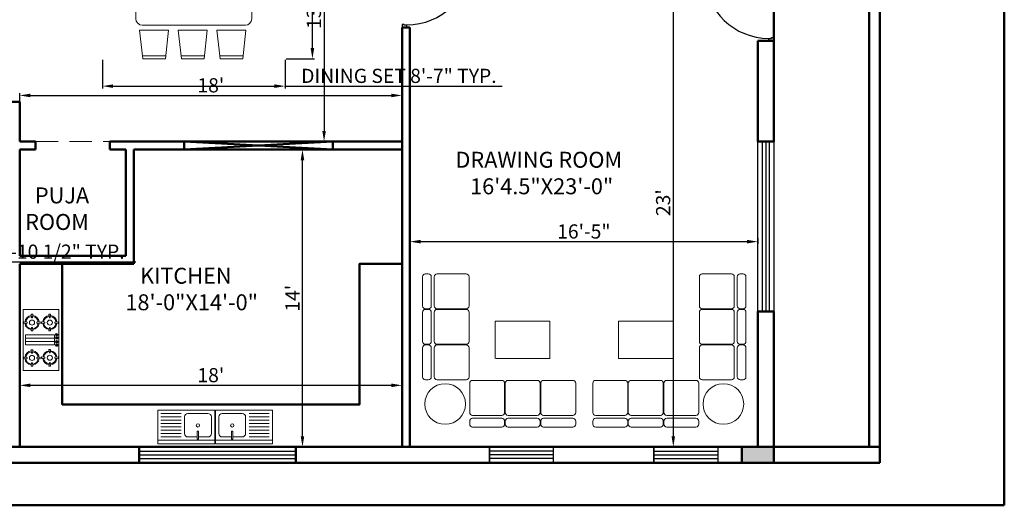
# Model space of a CAD drawing. Units: millimetres. Extents: x 1706 to 5913, y 156 to 1716.
# Tile 25 of 26: x 4935 to 5492, y 1141 to 1415. Entities that reach past the tile are written whole.
import ezdxf

# ---------------------------------------------------------------- set-up
doc = ezdxf.new("R2010")
doc.units = ezdxf.units.MM
doc.linetypes.add('DASHED', pattern=[19.05, 12.7, -6.35])
for name, color, linetype, lineweight in [('A-ANNO-DIMS', 2, 'Continuous', 18), ('A-AREA-IDEN', 3, 'Continuous', 18), ('A-COLS', 20, 'Continuous', 50), ('A-DOOR', 4, 'Continuous', 25), ('A-FLOR-OVHD', 9, 'DASHED', 18), ('A-FURN', 8, 'Continuous', 18), ('A-GLAZ', 150, 'Continuous', 25), ('A-WALL', 7, 'Continuous', 50)]:
    doc.layers.add(name, color=color, linetype=linetype, lineweight=lineweight)
doc.styles.get("Standard").update_dxf_attribs({"font": 'arial.ttf'})
doc.dimstyles.new('ISO-25', dxfattribs={"dimtxt": 8, "dimasz": 6, "dimexe": 1.25, "dimexo": 0.625, "dimtad": 1, "dimdec": 0, "dimlunit": 3, "dimtxsty": 'Standard', "dimcen": 2.5, "dimadec": 0, "dimazin": 0, "dimtfac": 1, "dimtdec": 0, "dimtmove": 0, "dimatfit": 3, "dimfxl": 1, "dimarcsym": 0})

# ---------------------------------------------------------------- blocks, each defined once
blk = doc.blocks.new('Puerta 01')
for p, q in [((-0.775, -0.026), (-0.737, -0.058)), ((-0.775, -0.058), (-0.737, -0.026)), ((-0.737, -0.058), (-0.737, -0.026)), ((-0.028, -0.058), (-0.066, -0.026)), ((-0.028, -0.026), (-0.066, -0.058)), ((-0.066, -0.058), (-0.066, -0.026))]:
    blk.add_line(p, q)
for points in [[(-0.028, 0), (-0.028, -0.026), (0.004, -0.026), (0.004, -0.036), (0.028, -0.036), (0.028, 0)], [(-0.028, -0.026), (-0.775, -0.026), (-0.775, -0.058), (-0.028, -0.058)], [(0.004, -0.774), (0.004, -0.764), (0.028, -0.764), (0.028, -0.8), (-0.028, -0.8), (-0.028, -0.774)]]:
    blk.add_lwpolyline(points, close=True)
blk.add_arc((-0.028, -0.026), 0.747, 182.4545, 270)
blk = doc.blocks.new('A$C57CF26DA')
for p, q in [((0, 0), (0, 420)), ((720, 420), (0, 420)), ((167, 413), (147, 413)), ((147, 413), (152, 373)), ((152, 373), (162, 373)), ((162, 373), (167, 413)), ((300, 391), (300, 49)), ((300, 391), (420, 391)), ((340, 391), (340, 49)), ((380, 391), (380, 49)), ((420, 391), (420, 49)), ((584, 413), (564, 413)), ((564, 413), (569, 373)), ((569, 373), (579, 373)), ((579, 373), (584, 413)), ((720, 0), (720, 420)), ((99, 320), (59, 325)), ((59, 325), (59, 305)), ((59, 305), (99, 310)), ((99, 310), (99, 320)), ((152, 257), (147, 217)), ((162, 257), (152, 257)), ((167, 217), (162, 257)), ((255, 325), (215, 320)), ((215, 320), (215, 310)), ((215, 310), (255, 305)), ((255, 305), (255, 325)), ((516, 320), (476, 325)), ((476, 325), (476, 305)), ((476, 305), (516, 310)), ((516, 310), (516, 320)), ((569, 257), (564, 217)), ((579, 257), (569, 257)), ((584, 217), (579, 257)), ((672, 325), (632, 320)), ((632, 320), (632, 310)), ((632, 310), (672, 305)), ((672, 305), (672, 325)), ((147, 217), (167, 217)), ((167, 203), (147, 203)), ((147, 203), (152, 163)), ((152, 163), (162, 163)), ((162, 163), (167, 203)), ((581, 203), (561, 203)), ((561, 203), (566, 163)), ((564, 217), (584, 217)), ((566, 163), (576, 163)), ((576, 163), (581, 203)), ((99, 110), (59, 115)), ((59, 115), (59, 95)), ((59, 95), (99, 100)), ((99, 100), (99, 110)), ((152, 47), (147, 7)), ((147, 7), (167, 7)), ((162, 47), (152, 47)), ((167, 7), (162, 47)), ((255, 115), (215, 110)), ((215, 110), (215, 100)), ((215, 100), (255, 95)), ((255, 95), (255, 115)), ((302, 39), (295, 39)), ((295, 39), (295, 11)), ((295, 11), (302, 11)), ((420, 49), (300, 49)), ((302, 11), (302, 39)), ((341, 39), (334, 39)), ((334, 39), (334, 11)), ((334, 11), (341, 11)), ((341, 11), (341, 39)), ((380, 11), (380, 39)), ((380, 39), (386, 39)), ((386, 11), (380, 11)), ((386, 39), (386, 11)), ((419, 11), (419, 39)), ((419, 39), (426, 39)), ((426, 11), (419, 11)), ((426, 39), (426, 11)), ((513, 110), (473, 115)), ((473, 115), (473, 95)), ((473, 95), (513, 100)), ((513, 100), (513, 110)), ((566, 47), (561, 7)), ((561, 7), (581, 7)), ((576, 47), (566, 47)), ((581, 7), (576, 47)), ((669, 115), (629, 110)), ((629, 110), (629, 100)), ((629, 100), (669, 95)), ((669, 95), (669, 115)), ((720, 0), (0, 0))]:
    blk.add_line(p, q)
for centre in [(157, 315), (574, 315), (157, 105), (571, 105)]:
    blk.add_circle(centre, 30)
for centre, radius, start, end in [((157, 315), 83, 95.5849, 174.4151), ((157, 315), 73, 95.3738, 174.6262), ((157, 315), 73, 5.3738, 84.6262), ((157, 315), 83, 5.5849, 84.4151), ((574, 315), 83, 95.5849, 174.4151), ((574, 315), 73, 95.3738, 174.6262), ((574, 315), 73, 5.3738, 84.6262), ((574, 315), 83, 5.5849, 84.4151), ((157, 315), 83, 185.5849, 264.4151), ((157, 315), 73, 185.3738, 264.6262), ((157, 315), 73, 275.3738, 354.6262), ((157, 315), 83, 275.5849, 354.4151), ((574, 315), 83, 185.5849, 264.4151), ((574, 315), 73, 185.3738, 264.6262), ((574, 315), 73, 275.3738, 354.6262), ((574, 315), 83, 275.5849, 354.4151), ((157, 105), 83, 95.5849, 174.4151), ((157, 105), 73, 95.3738, 174.6262), ((157, 105), 73, 5.3738, 84.6262), ((157, 105), 83, 5.5849, 84.4151), ((571, 105), 83, 95.5849, 174.4151), ((571, 105), 73, 95.3738, 174.6262), ((571, 105), 73, 5.3738, 84.6262), ((571, 105), 83, 5.5849, 84.4151), ((157, 105), 83, 185.5849, 264.4151), ((157, 105), 73, 185.3738, 264.6262), ((157, 105), 73, 275.3738, 354.6262), ((157, 105), 83, 275.5849, 354.4151), ((298, 25), 13.7, 104.4775, 255.5225), ((298, 25), 13.7, 284.4775, 75.5225), ((337, 25), 13.7, 104.4775, 255.5225), ((337, 25), 13.7, 284.4775, 75.5225), ((383, 25), 13.7, 104.4775, 255.5225), ((383, 25), 13.7, 284.4775, 75.5225), ((422, 25), 13.7, 104.4775, 255.5225), ((422, 25), 13.7, 284.4775, 75.5225), ((571, 105), 83, 185.5849, 264.4151), ((571, 105), 73, 185.3738, 264.6262), ((571, 105), 73, 275.3738, 354.6262), ((571, 105), 83, 275.5849, 354.4151)]:
    blk.add_arc(centre, radius, start, end)
blk = doc.blocks.new('A$C3404121D')
for p, q in [((0, 0), (0, 500)), ((0, 500), (850, 500)), ((0, 450), (850, 450)), ((850, 500), (850, 0)), ((50, 100), (50, 350)), ((100, 400), (240, 400)), ((240, 431), (240, 425)), ((260, 431), (240, 431)), ((240, 425), (240, 315)), ((240, 315), (260, 315)), ((260, 431), (260, 315)), ((260, 400), (400, 400)), ((450, 100), (450, 350)), ((502, 400), (801, 400)), ((502, 350), (801, 350)), ((502, 300), (801, 300)), ((502, 250), (801, 250)), ((502, 200), (801, 200)), ((502, 150), (801, 150)), ((850, 0), (0, 0)), ((400, 50), (100, 50)), ((502, 100), (801, 100)), ((801, 50), (502, 50))]:
    blk.add_line(p, q)
blk.add_circle((250, 228), 25)
for centre, start, end in [((100, 350), 90, 180), ((400, 350), 0, 90), ((100, 100), 180, 270), ((400, 100), 270, 0)]:
    blk.add_arc(centre, 50, start, end)
blk = doc.blocks.new('A$C59D7588A')
for p, q in [((0.575, 1.5), (0.623, 1.943)), ((0.618, 1.9), (0.982, 1.9)), ((0.623, 1.943), (0.978, 1.943)), ((0.978, 1.943), (1.025, 1.5)), ((1.175, 1.5), (1.223, 1.943)), ((1.218, 1.9), (1.582, 1.9)), ((1.223, 1.943), (1.578, 1.943)), ((1.578, 1.943), (1.625, 1.5)), ((1.775, 1.5), (1.823, 1.943)), ((1.818, 1.9), (2.182, 1.9)), ((1.823, 1.943), (2.178, 1.943)), ((2.178, 1.943), (2.225, 1.5)), ((1.025, 1.5), (0.575, 1.5)), ((0.616, 1.421), (2.216, 1.421)), ((1.625, 1.5), (1.175, 1.5)), ((2.225, 1.5), (1.775, 1.5)), ((0.516, 0.621), (0.516, 1.321)), ((2.316, 1.321), (2.316, 0.621)), ((0, 1.146), (0.443, 1.194)), ((0, 0.792), (0, 1.146)), ((0.043, 0.787), (0.043, 1.151)), ((0.443, 1.194), (0.443, 0.744)), ((2.832, 1.146), (2.389, 1.194)), ((2.389, 1.194), (2.389, 0.744)), ((2.789, 0.787), (2.789, 1.151)), ((2.832, 0.792), (2.832, 1.146)), ((0.443, 0.744), (0, 0.792)), ((2.389, 0.744), (2.832, 0.792)), ((2.216, 0.521), (0.616, 0.521)), ((1.025, 0.443), (0.575, 0.443)), ((0.575, 0.443), (0.623, 0)), ((0.978, 0), (1.025, 0.443)), ((1.625, 0.443), (1.175, 0.443)), ((1.175, 0.443), (1.223, 0)), ((1.578, 0), (1.625, 0.443)), ((2.225, 0.443), (1.775, 0.443)), ((1.775, 0.443), (1.823, 0)), ((2.178, 0), (2.225, 0.443)), ((0.618, 0.043), (0.982, 0.043)), ((1.218, 0.043), (1.582, 0.043)), ((1.818, 0.043), (2.182, 0.043)), ((0.623, 0), (0.978, 0)), ((1.223, 0), (1.578, 0)), ((1.823, 0), (2.178, 0))]:
    blk.add_line(p, q)
for centre, start, end in [((0.616, 1.321), 90, 180), ((2.216, 1.321), 0, 90), ((0.616, 0.621), 180, 270), ((2.216, 0.621), 270, 0)]:
    blk.add_arc(centre, 0.1, start, end)
blk = doc.blocks.new('A$C753D6792')
at = {"linetype": 'ByBlock'}
for p, q in [((0, 2530), (0, 2580)), ((50, 2630), (550, 2630)), ((600, 2580), (600, 2530)), ((610, 2530), (610, 2580)), ((660, 2630), (1160, 2630)), ((1210, 2580), (1210, 2530)), ((1220, 2530), (1220, 2580)), ((1270, 2630), (1770, 2630)), ((1820, 2580), (1820, 2530)), ((0, 1880), (0, 2380)), ((550, 2480), (50, 2480)), ((550, 2430), (50, 2430)), ((600, 2380), (600, 1880)), ((610, 1880), (610, 2380)), ((1160, 2480), (660, 2480)), ((1160, 2430), (660, 2430)), ((1210, 2380), (1210, 1880)), ((1220, 1880), (1220, 2380)), ((1770, 2480), (1270, 2480)), ((1770, 2430), (1270, 2430)), ((1820, 1880), (1820, 2380)), ((50, 1830), (427, 1830)), ((387, 1830), (550, 1830)), ((660, 1830), (1037, 1830)), ((997, 1830), (1160, 1830)), ((1270, 1830), (1647, 1830)), ((1607, 1830), (1770, 1830)), ((1830, 1770), (1830, 1393)), ((1880, 1820), (2380, 1820)), ((2430, 1270), (2430, 1770)), ((2480, 1270), (2480, 1770)), ((2530, 1820), (2580, 1820)), ((2630, 1770), (2630, 1270)), ((442, 815), (442, 1455)), ((442, 1455), (1372, 1455)), ((1382, 1455), (1382, 815)), ((1830, 1433), (1830, 1270)), ((2380, 1220), (1880, 1220)), ((1880, 1210), (2380, 1210)), ((2580, 1220), (2530, 1220)), ((2530, 1210), (2580, 1210)), ((1830, 1160), (1830, 783)), ((2430, 660), (2430, 1160)), ((2480, 660), (2480, 1160)), ((2630, 1160), (2630, 660)), ((1382, 815), (442, 815)), ((1830, 823), (1830, 660)), ((1830, 550), (1830, 173)), ((2380, 610), (1880, 610)), ((1880, 600), (2380, 600)), ((2430, 50), (2430, 550)), ((2480, 50), (2480, 550)), ((2580, 610), (2530, 610)), ((2530, 600), (2580, 600)), ((2630, 550), (2630, 50)), ((1830, 213), (1830, 50)), ((2380, 0), (1880, 0)), ((2580, 0), (2530, 0))]:
    blk.add_line(p, q, dxfattribs=at)
blk.add_circle((2242, 2235), 349, dxfattribs=at)
for centre, start, end in [((50, 2580), 90, 180), ((550, 2580), 0, 90), ((550, 2580), 0, 90), ((660, 2580), 90, 180), ((1160, 2580), 0, 90), ((1160, 2580), 0, 90), ((1270, 2580), 90, 180), ((1770, 2580), 0, 90), ((1770, 2580), 0, 90), ((50, 2530), 180, 270), ((50, 2380), 90, 180), ((550, 2530), 270, 0), ((550, 2530), 270, 0), ((550, 2380), 0, 90), ((550, 2380), 0, 90), ((660, 2530), 180, 270), ((660, 2380), 90, 180), ((1160, 2530), 270, 0), ((1160, 2530), 270, 0), ((1160, 2380), 0, 90), ((1160, 2380), 0, 90), ((1270, 2530), 180, 270), ((1270, 2380), 90, 180), ((1770, 2530), 270, 0), ((1770, 2530), 270, 0), ((1770, 2380), 0, 90), ((1770, 2380), 0, 90), ((50, 1880), 180, 270), ((550, 1880), 270, 0), ((660, 1880), 180, 270), ((1160, 1880), 270, 0), ((1270, 1880), 180, 270), ((1770, 1880), 270, 0), ((1880, 1770), 90, 180), ((2380, 1770), 0, 90), ((2530, 1770), 90, 180), ((2580, 1770), 0, 90), ((1880, 1270), 180, 270), ((1880, 1160), 90, 180), ((2380, 1270), 270, 0), ((2380, 1270), 270, 0), ((2380, 1160), 0, 90), ((2530, 1270), 180, 270), ((2530, 1270), 180, 270), ((2530, 1160), 90, 180), ((2580, 1270), 270, 0), ((2580, 1270), 270, 0), ((2580, 1160), 0, 90), ((1880, 660), 180, 270), ((1880, 550), 90, 180), ((2380, 660), 270, 0), ((2380, 660), 270, 0), ((2380, 550), 0, 90), ((2530, 660), 180, 270), ((2530, 660), 180, 270), ((2530, 550), 90, 180), ((2580, 660), 270, 0), ((2580, 660), 270, 0), ((2580, 550), 0, 90), ((1880, 50), 180, 270), ((2380, 50), 270, 0), ((2380, 50), 270, 0), ((2530, 50), 180, 270), ((2530, 50), 180, 270), ((2580, 50), 270, 0), ((2580, 50), 270, 0)]:
    blk.add_arc(centre, 50, start, end, dxfattribs=at)
blk = doc.blocks.new('*D68')
at = {"layer": 'A-ANNO-DIMS', "color": 0, "lineweight": -2, "transparency": 16777216}
for p, q in [((5104.76, 1503.68), (5108.61, 1503.68)), ((5107.36, 1497.68), (5107.36, 1352.18)), ((5104.76, 1346.18), (5108.61, 1346.18))]:
    blk.add_line(p, q, dxfattribs=at)
at = {"layer": 'A-ANNO-DIMS', "color": 0, "transparency": 16777216}
for points in [[(5106.36, 1497.68), (5108.36, 1497.68), (5107.36, 1503.68)], [(5106.36, 1352.18), (5108.36, 1352.18), (5107.36, 1346.18)]]:
    blk.add_solid(points, dxfattribs=at)
at = {"layer": 'Defpoints', "color": 0, "transparency": 16777216}
for p in [(5104.13, 1503.68), (5104.13, 1346.18), (5107.36, 1346.18)]:
    blk.add_point(p, dxfattribs=at)
at = {"layer": 'A-ANNO-DIMS', "color": 0, "transparency": 16777216, "insert": (5102.64, 1424.93), "char_height": 8, "attachment_point": 5, "rotation": 90}
blk.add_mtext('13\'-2"', dxfattribs=at)
blk = doc.blocks.new('*D69')
at = {"layer": 'A-ANNO-DIMS', "color": 0, "lineweight": -2, "transparency": 16777216}
for p, q in [((4935.38, 1359.93), (4935.38, 1373.5)), ((4941.38, 1372.25), (5145.38, 1372.25)), ((5151.38, 1359.93), (5151.38, 1373.5))]:
    blk.add_line(p, q, dxfattribs=at)
at = {"layer": 'A-ANNO-DIMS', "color": 0, "transparency": 16777216}
for points in [[(4941.38, 1373.25), (4941.38, 1371.25), (4935.38, 1372.25)], [(5145.38, 1373.25), (5145.38, 1371.25), (5151.38, 1372.25)]]:
    blk.add_solid(points, dxfattribs=at)
at = {"layer": 'Defpoints', "color": 0, "transparency": 16777216}
for p in [(5151.38, 1372.25), (4935.38, 1359.3), (5151.38, 1359.3)]:
    blk.add_point(p, dxfattribs=at)
at = {"layer": 'A-ANNO-DIMS', "color": 0, "transparency": 16777216, "insert": (5043.38, 1376.96), "char_height": 8, "attachment_point": 5}
blk.add_mtext("18'", dxfattribs=at)
blk = doc.blocks.new('*D70')
at = {"layer": 'A-ANNO-DIMS', "color": 0, "lineweight": -2, "transparency": 16777216}
for p, q in [((5096.14, 1341.68), (5093.9, 1341.68)), ((5095.15, 1179.68), (5095.15, 1335.68)), ((5096.14, 1173.68), (5093.9, 1173.68))]:
    blk.add_line(p, q, dxfattribs=at)
at = {"layer": 'A-ANNO-DIMS', "color": 0, "transparency": 16777216}
for points in [[(5094.15, 1335.68), (5096.15, 1335.68), (5095.15, 1341.68)], [(5094.15, 1179.68), (5096.15, 1179.68), (5095.15, 1173.68)]]:
    blk.add_solid(points, dxfattribs=at)
at = {"layer": 'Defpoints', "color": 0, "transparency": 16777216}
for p in [(5095.15, 1341.68), (5096.77, 1341.68), (5096.77, 1173.68)]:
    blk.add_point(p, dxfattribs=at)
at = {"layer": 'A-ANNO-DIMS', "color": 0, "transparency": 16777216, "insert": (5090.51, 1257.68), "char_height": 8, "attachment_point": 5, "rotation": 90}
blk.add_mtext("14'", dxfattribs=at)
blk = doc.blocks.new('*D71')
at = {"layer": 'A-ANNO-DIMS', "color": 0, "lineweight": -2, "transparency": 16777216}
for p, q in [((4935.38, 1201.14), (4935.38, 1209.73)), ((4941.38, 1208.48), (5145.38, 1208.48)), ((5151.38, 1201.14), (5151.38, 1209.73))]:
    blk.add_line(p, q, dxfattribs=at)
at = {"layer": 'A-ANNO-DIMS', "color": 0, "transparency": 16777216}
for points in [[(4941.38, 1209.48), (4941.38, 1207.48), (4935.38, 1208.48)], [(5145.38, 1209.48), (5145.38, 1207.48), (5151.38, 1208.48)]]:
    blk.add_solid(points, dxfattribs=at)
at = {"layer": 'Defpoints', "color": 0, "transparency": 16777216}
for p in [(5151.38, 1208.48), (4935.38, 1200.51), (5151.38, 1200.51)]:
    blk.add_point(p, dxfattribs=at)
at = {"layer": 'A-ANNO-DIMS', "color": 0, "transparency": 16777216, "insert": (5043.38, 1213.19), "char_height": 8, "attachment_point": 5}
blk.add_mtext("18'", dxfattribs=at)
blk = doc.blocks.new('*D72')
at = {"layer": 'A-ANNO-DIMS', "color": 0, "lineweight": -2, "transparency": 16777216}
for p, q in [((5301.19, 1449.68), (5305.91, 1449.68)), ((5304.66, 1443.68), (5304.66, 1179.68)), ((5301.19, 1173.68), (5305.91, 1173.68))]:
    blk.add_line(p, q, dxfattribs=at)
at = {"layer": 'A-ANNO-DIMS', "color": 0, "transparency": 16777216}
for points in [[(5303.66, 1443.68), (5305.66, 1443.68), (5304.66, 1449.68)], [(5303.66, 1179.68), (5305.66, 1179.68), (5304.66, 1173.68)]]:
    blk.add_solid(points, dxfattribs=at)
at = {"layer": 'Defpoints', "color": 0, "transparency": 16777216}
for p in [(5300.56, 1449.68), (5300.56, 1173.68), (5304.66, 1173.68)]:
    blk.add_point(p, dxfattribs=at)
at = {"layer": 'A-ANNO-DIMS', "color": 0, "transparency": 16777216, "insert": (5299.95, 1311.68), "char_height": 8, "attachment_point": 5, "rotation": 90}
blk.add_mtext("23'", dxfattribs=at)
blk = doc.blocks.new('*D73')
at = {"layer": 'A-ANNO-DIMS', "color": 0, "lineweight": -2, "transparency": 16777216}
for p, q in [((5155.88, 1291.56), (5155.88, 1288.41)), ((5352.38, 1291.56), (5352.38, 1288.41)), ((5161.88, 1289.66), (5346.38, 1289.66))]:
    blk.add_line(p, q, dxfattribs=at)
at = {"layer": 'A-ANNO-DIMS', "color": 0, "transparency": 16777216}
for points in [[(5161.88, 1290.66), (5161.88, 1288.66), (5155.88, 1289.66)], [(5346.38, 1290.66), (5346.38, 1288.66), (5352.38, 1289.66)]]:
    blk.add_solid(points, dxfattribs=at)
at = {"layer": 'Defpoints', "color": 0, "transparency": 16777216}
for p in [(5155.88, 1292.18), (5352.38, 1292.18), (5352.38, 1289.66)]:
    blk.add_point(p, dxfattribs=at)
at = {"layer": 'A-ANNO-DIMS', "color": 0, "transparency": 16777216, "insert": (5254.13, 1294.37), "char_height": 8, "attachment_point": 5}
blk.add_mtext('16\'-5"', dxfattribs=at)
blk = doc.blocks.new('*D215')
at = {"layer": 'A-ANNO-DIMS', "color": 0, "lineweight": -2, "transparency": 16777216}
for p, q in [((4692.95, 1264.63), (4692.95, 1279.45)), ((4698.95, 1278.2), (4781.6, 1278.2)), ((4787.6, 1264.63), (4787.6, 1279.45)), ((4787.6, 1278.2), (5001.01, 1278.2))]:
    blk.add_line(p, q, dxfattribs=at)
at = {"layer": 'A-ANNO-DIMS', "color": 0, "transparency": 16777216}
for points in [[(4698.95, 1279.2), (4698.95, 1277.2), (4692.95, 1278.2)], [(4781.6, 1279.2), (4781.6, 1277.2), (4787.6, 1278.2)]]:
    blk.add_solid(points, dxfattribs=at)
at = {"layer": 'Defpoints', "color": 0, "transparency": 16777216}
for p in [(4787.6, 1278.2), (4692.95, 1264.01), (4787.6, 1264.01)]:
    blk.add_point(p, dxfattribs=at)
at = {"layer": 'A-ANNO-DIMS', "color": 0, "transparency": 16777216, "insert": (4897.3, 1282.96), "char_height": 8, "attachment_point": 5}
blk.add_mtext('BED WITH SIDE TABLES 7\'-10 1/2" TYP.', dxfattribs=at)
blk = doc.blocks.new('*D231')
at = {"layer": 'A-ANNO-DIMS', "color": 0, "lineweight": -2, "transparency": 16777216}
for p, q in [((4982.19, 1392.37), (4982.19, 1376.27)), ((5085.29, 1392.37), (5085.29, 1376.27)), ((4988.19, 1377.52), (5079.29, 1377.52)), ((5085.29, 1377.52), (5207.97, 1377.52))]:
    blk.add_line(p, q, dxfattribs=at)
at = {"layer": 'A-ANNO-DIMS', "color": 0, "transparency": 16777216}
for points in [[(4988.19, 1378.52), (4988.19, 1376.52), (4982.19, 1377.52)], [(5079.29, 1378.52), (5079.29, 1376.52), (5085.29, 1377.52)]]:
    blk.add_solid(points, dxfattribs=at)
at = {"layer": 'Defpoints', "color": 0, "transparency": 16777216}
for p in [(4982.19, 1392.99), (5085.29, 1392.99), (5085.29, 1377.52)]:
    blk.add_point(p, dxfattribs=at)
at = {"layer": 'A-ANNO-DIMS', "color": 0, "transparency": 16777216, "insert": (5149.63, 1382.29), "char_height": 8, "attachment_point": 5}
blk.add_mtext('DINING SET 8\'-7" TYP.', dxfattribs=at)
blk = doc.blocks.new('*D232')
at = {"layer": 'A-ANNO-DIMS', "color": 0, "lineweight": -2, "transparency": 16777216}
for p, q in [((5100.76, 1463.72), (5100.76, 1544.6)), ((5085.92, 1463.72), (5102.01, 1463.72)), ((5100.76, 1398.99), (5100.76, 1457.72)), ((5085.92, 1392.99), (5102.01, 1392.99))]:
    blk.add_line(p, q, dxfattribs=at)
at = {"layer": 'A-ANNO-DIMS', "color": 0, "transparency": 16777216}
for points in [[(5099.76, 1457.72), (5101.76, 1457.72), (5100.76, 1463.72)], [(5099.76, 1398.99), (5101.76, 1398.99), (5100.76, 1392.99)]]:
    blk.add_solid(points, dxfattribs=at)
at = {"layer": 'Defpoints', "color": 0, "transparency": 16777216}
for p in [(5085.29, 1463.72), (5100.76, 1463.72), (5085.29, 1392.99)]:
    blk.add_point(p, dxfattribs=at)
at = {"layer": 'A-ANNO-DIMS', "color": 0, "transparency": 16777216, "insert": (5096, 1507.16), "char_height": 8, "attachment_point": 5, "rotation": 90}
blk.add_mtext('5\'-10 1/2" TYP.', dxfattribs=at)

msp = doc.modelspace()

# ---------------------------------------------------------------- hatches: boundary and pattern name
at = {"layer": 'A-COLS'}
h = msp.add_hatch(color=256, dxfattribs=at)
h.dxf.hatch_style = 1
h.paths.add_polyline_path([(5361.38, 1173.68), (5343.38, 1173.68), (5343.38, 1164.68), (5361.38, 1164.68)])

# ---------------------------------------------------------------- linework, layer by layer
msp.add_lwpolyline([(5361.6, 1173.68), (5343.38, 1173.68), (5343.38, 1164.68), (5361.38, 1164.68), (5361.38, 1173.68)], dxfattribs=at)
at = {"layer": 'A-FLOR-OVHD'}
msp.add_line((4944.38, 1346.18), (4986.38, 1346.18), dxfattribs=at)
at = {"layer": 'A-GLAZ'}
for p, q in [((5354.88, 1346.18), (5354.88, 1250.18)), ((5356.88, 1346.18), (5356.88, 1250.18)), ((5358.88, 1346.18), (5358.88, 1250.18)), ((5002.88, 1171.18), (5091.38, 1171.18)), ((5002.88, 1169.18), (5091.38, 1169.18)), ((5200.74, 1173.68), (5200.74, 1164.68)), ((5236.74, 1171.18), (5200.74, 1171.18)), ((5236.74, 1169.18), (5200.74, 1169.18)), ((5236.74, 1173.68), (5236.74, 1164.68)), ((5293.74, 1173.68), (5293.74, 1164.68)), ((5293.74, 1171.18), (5329.74, 1171.18)), ((5293.74, 1169.18), (5329.74, 1169.18)), ((5329.74, 1173.68), (5329.74, 1164.68)), ((5002.88, 1167.18), (5091.38, 1167.18)), ((5236.74, 1167.18), (5200.74, 1167.18)), ((5293.74, 1167.18), (5329.74, 1167.18))]:
    msp.add_line(p, q, dxfattribs=at)
for points in [[(5352.38, 1346.18), (5361.38, 1346.18), (5361.38, 1250.18), (5352.38, 1250.18)], [(5002.88, 1173.68), (5091.38, 1173.68), (5091.38, 1164.68), (5002.88, 1164.68)], [(5200.74, 1173.68), (5236.74, 1173.68), (5236.74, 1164.68), (5200.74, 1164.68)], [(5293.74, 1173.68), (5329.74, 1173.68), (5329.74, 1164.68), (5293.74, 1164.68)]]:
    msp.add_lwpolyline(points, close=True, dxfattribs=at)
at = {"layer": 'A-WALL'}
for p, q in [((5491.67, 1664.18), (5491.67, 1140.68)), ((5415.38, 1655.18), (5415.38, 1173.68)), ((5421.38, 1655.18), (5421.38, 1173.68)), ((5361.38, 1442.18), (5361.38, 1403.18)), ((5151.38, 1410.68), (5151.38, 1173.68)), ((5151.38, 1410.68), (5155.88, 1410.68)), ((5155.88, 1410.68), (5155.88, 1173.68)), ((5352.38, 1403.18), (5352.38, 1346.18)), ((5361.38, 1403.18), (5352.38, 1403.18)), ((5361.38, 1403.18), (5361.38, 1346.18)), ((4930.88, 1368.68), (4935.38, 1368.68)), ((4935.38, 1368.68), (4935.38, 1346.18)), ((4935.38, 1346.18), (4944.38, 1346.18)), ((4935.38, 1341.68), (4935.38, 1281.68)), ((4935.38, 1341.68), (4944.38, 1341.68)), ((4944.38, 1346.18), (4944.38, 1341.68)), ((4986.38, 1346.18), (4986.38, 1341.68)), ((4986.38, 1346.18), (5028.38, 1346.18)), ((4986.38, 1341.68), (4995.38, 1341.68)), ((4995.38, 1341.68), (4995.38, 1281.68)), ((4999.88, 1341.68), (4999.88, 1277.18)), ((4999.88, 1341.68), (5028.38, 1341.68)), ((5028.38, 1346.18), (5028.38, 1341.68)), ((5112.38, 1346.18), (5028.38, 1341.68)), ((5028.38, 1346.18), (5112.38, 1341.68)), ((5112.38, 1346.18), (5112.38, 1341.68)), ((5112.38, 1346.18), (5151.38, 1346.18)), ((5112.38, 1341.68), (5151.38, 1341.68)), ((5361.38, 1346.18), (5352.38, 1346.18)), ((4935.38, 1281.68), (4995.38, 1281.68)), ((4935.38, 1277.18), (4935.38, 1173.68)), ((4935.38, 1277.18), (4999.88, 1277.18)), ((5352.38, 1250.18), (5352.38, 1173.68)), ((5361.38, 1250.18), (5352.38, 1250.18)), ((5361.38, 1250.18), (5361.38, 1173.68)), ((4626.38, 1173.68), (5421.38, 1173.68)), ((5002.88, 1173.68), (5002.88, 1164.68)), ((5091.38, 1173.68), (5091.38, 1164.68)), ((5361.38, 1173.68), (5361.38, 1164.68)), ((5361.38, 1164.68), (5361.38, 1173.68)), ((5421.38, 1173.68), (5421.38, 1164.68)), ((4621.88, 1164.68), (5421.38, 1164.68)), ((4596.38, 1140.68), (5491.67, 1140.68))]:
    msp.add_line(p, q, dxfattribs=at)
msp.add_lwpolyline([(5028.38, 1346.18), (5112.38, 1346.18), (5112.38, 1341.68), (5028.38, 1341.68)], close=True, dxfattribs=at)
msp.add_lwpolyline([(4959.38, 1277.18), (4959.38, 1197.68), (5127.38, 1197.68), (5127.38, 1277.18), (5151.38, 1277.18)], dxfattribs=at)

# ---------------------------------------------------------------- block references
at = {"layer": 'A-DOOR', "yscale": 48.75000000000287, "zscale": 48.75000000000287}
for p, xscale in [((5152.75, 1449.68), -48.75000000000287), ((5360.02, 1442.18), 48.75000000000287)]:
    msp.add_blockref('Puerta 01', p, dxfattribs=dict(at, xscale=xscale))
at = {"layer": 'A-FURN', "xscale": 36.4071025162376, "yscale": 36.4071025162376, "zscale": 36.4071025162376}
msp.add_blockref('A$C59D7588A', (4982.19, 1392.99), dxfattribs=at)
at = {"layer": 'A-FURN'}
for name, p, xscale, yscale, zscale, rotation in [('A$C753D6792', (5249.5, 1271.46), 0.0329035460231199, 0.0329035460231199, 0.0329035460231199, 180), ('A$C753D6792', (5259.18, 1271.46), -0.0329035460231199, 0.0329035460231199, 0.0329035460231199, 180), ('A$C57CF26DA', (4957.42, 1251.41), -0.0478777176975714, 0.0478777176975714, 0.0478777176975714, 90), ('A$C3404121D', (5045.56, 1194.45), 0.0378984485580132, 0.0378984485580132, 0.0378984485580132, 180), ('A$C3404121D', (5045.97, 1194.45), -0.0378984485580132, 0.0378984485580132, 0.0378984485580132, 180)]:
    msp.add_blockref(name, p, dxfattribs=dict(at, xscale=xscale, yscale=yscale, zscale=zscale, rotation=rotation))

# ---------------------------------------------------------------- texts
at = {"layer": 'A-AREA-IDEN', "char_height": 9, "attachment_point": 1}
for s, width, insert in [('    DRAWING ROOM\\P       16\'4.5"X23\'-0"', 125.2434, (5170.59, 1340.43)), ('  PUJA ROOM', 67.9131, (4938.47, 1320.28)), ('    KITCHEN\\P 18\'-0"X14\'-0"', 99.443, (4992.34, 1274.89))]:
    msp.add_mtext_dynamic_manual_height_columns(s, width=width, gutter_width=12.5, heights=[0], dxfattribs=dict(at, insert=insert))

# ---------------------------------------------------------------- dimensions: what is measured, and where the dimension line sits
at = {"layer": 'A-ANNO-DIMS'}
dim = msp.add_linear_dim(base=(5100.76, 1463.72), p1=(5085.29, 1392.99), p2=(5085.29, 1463.72), angle=90, text='<> TYP.', dimstyle='ISO-25', override={"dimdec": 1, "dimrnd": 0, "dimzin": 1, "dimlunit": 4, "dimfrac": 2}, dxfattribs=at)
dim.commit()
dim.dimension.update_dxf_attribs({"geometry": '*D232', "text_midpoint": (5096, 1507.16)})
for base, p1, p2, picture, middle in [((5107.3562305, 1346.18004162), (5104.13109307, 1503.68004162), (5104.13109307, 1346.18004162), '*D68', (5102.64391809, 1424.93004162)), ((5304.66, 1173.68), (5300.56, 1449.68), (5300.56, 1173.68), '*D72', (5299.95, 1311.68)), ((5095.15, 1341.68), (5096.77, 1173.68), (5096.77, 1341.68), '*D70', (5090.51, 1257.68))]:
    dim = msp.add_linear_dim(base=base, p1=p1, p2=p2, angle=90, dimstyle='ISO-25', override={"dimclrd": 0, "dimclre": 0, "dimclrt": 0}, dxfattribs=at)
    dim.commit()
    dim.dimension.update_dxf_attribs({"geometry": picture, "text_midpoint": middle})
for base, p1, p2, text, picture, middle in [((5085.29, 1377.52), (4982.19, 1392.99), (5085.29, 1392.99), 'DINING SET <> TYP.', '*D231', (5149.63, 1382.29)), ((4787.5956, 1278.2023), (4692.9486, 1264.0053), (4787.5956, 1264.0053), 'BED WITH SIDE TABLES <> TYP.', '*D215', (4897.3011, 1282.9638))]:
    dim = msp.add_linear_dim(base=base, p1=p1, p2=p2, text=text, dimstyle='ISO-25', override={"dimdec": 1, "dimrnd": 0, "dimzin": 1, "dimlunit": 4, "dimfrac": 2}, dxfattribs=at)
    dim.commit()
    dim.dimension.update_dxf_attribs({"geometry": picture, "text_midpoint": middle})
for base, p1, p2, picture, middle in [((5151.38, 1372.25), (4935.38, 1359.3), (5151.38, 1359.3), '*D69', (5043.38, 1376.96)), ((5352.38109307, 1289.66249214), (5155.88109307, 1292.18004162), (5352.38109307, 1292.18004162), '*D73', (5254.13109307, 1294.37207604)), ((5151.38, 1208.48), (4935.38, 1200.51), (5151.38, 1200.51), '*D71', (5043.38, 1213.19))]:
    dim = msp.add_linear_dim(base=base, p1=p1, p2=p2, dimstyle='ISO-25', override={"dimclrd": 0, "dimclre": 0, "dimclrt": 0}, dxfattribs=at)
    dim.commit()
    dim.dimension.update_dxf_attribs({"geometry": picture, "text_midpoint": middle})

doc.saveas('drawing.dxf')
